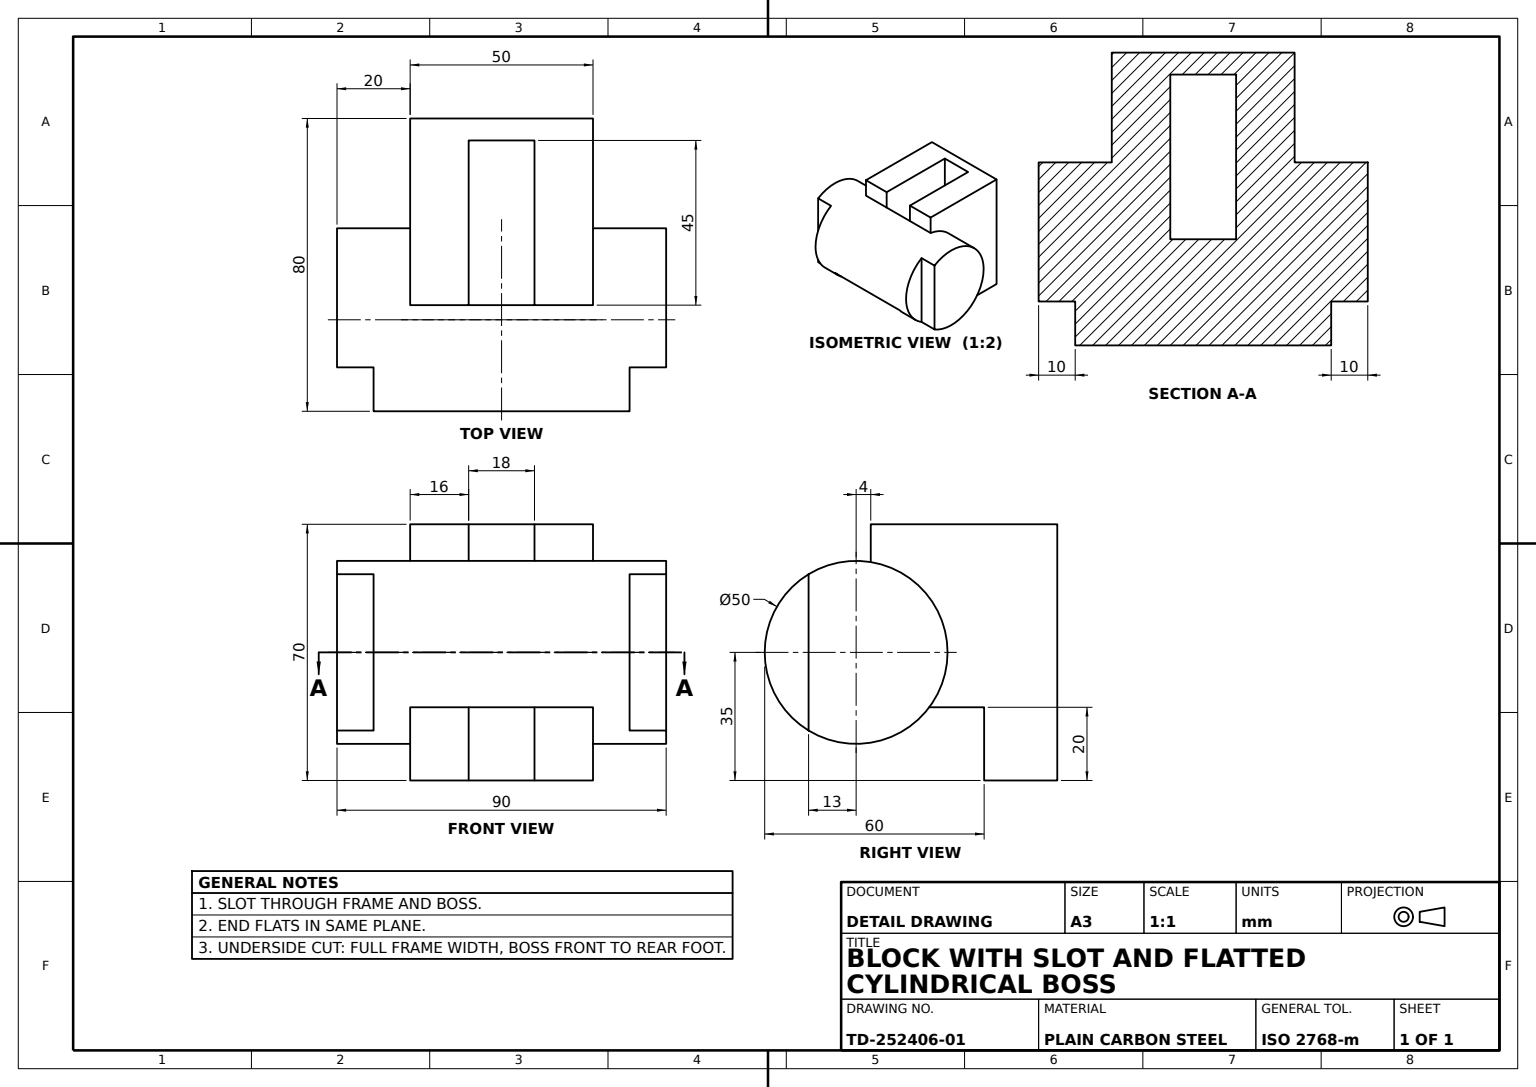
from build123d import *

# Parameters (mm, degrees)
BASE_PLATE_SKETCH_W         = 50
BASE_PLATE_SKETCH_H         = 70
BASE_PLATE_DEPTH            = 9
U_FRAME_SKETCH_W            = 16
U_FRAME_SKETCH_H            = 11
U_FRAME_DEPTH               = 70
SIDE_BLOCK_A_SKETCH_W       = 34
SIDE_BLOCK_A_SKETCH_H       = 50
SIDE_BLOCK_A_DEPTH          = 16
SIDE_BLOCK_B_SKETCH_W       = 34
SIDE_BLOCK_B_SKETCH_H       = 50
SIDE_BLOCK_B_DEPTH          = 16
BASE_RECESS_SKETCH_W        = 50
BASE_RECESS_SKETCH_H        = 70
BASE_RECESS_CUT_DEPTH       = 3
TOP_LIP_SKETCH_W            = 16
TOP_LIP_SKETCH_H            = 20
TOP_LIP_DEPTH               = 3
CYLINDER_SKETCH_R           = 25
CYLINDER_50_DEPTH           = 70
CYLINDER_START              = 20
CYLINDER_EXTENSION_SKETCH_R = 25
CYLINDER_EXTENSION_50_DEPTH = 20
U_SLOT_CUT_DEPTH            = 60
FRAME_CLEARANCE_SKETCH_W    = 18
FRAME_CLEARANCE_SKETCH_H    = 21
FRAME_CLEARANCE_CUT_DEPTH   = 50
END_FLAT_A_DEPTH            = 10
END_START                   = -10
END_FLAT_B_DEPTH            = 10


with BuildPart() as part:
    # Base Plate Sketch → Base Plate (new body)
    with BuildSketch(Plane.XY):
        with Locations((25, -35)):
            Rectangle(BASE_PLATE_SKETCH_W, BASE_PLATE_SKETCH_H)
    extrude(amount=BASE_PLATE_DEPTH)

    # U-Frame Sketch → U-Frame (add)
    with BuildSketch(Plane.XZ.offset(70)):
        with Locations((8, 14.5)):
            Rectangle(U_FRAME_SKETCH_W, U_FRAME_SKETCH_H)
        with Locations((42, 14.5)):
            Rectangle(U_FRAME_SKETCH_W, U_FRAME_SKETCH_H)
    extrude(amount=-U_FRAME_DEPTH)

    # Side Block A Sketch → Side Block A (add)
    with BuildSketch(Plane.ZY):
        with Locations((37, -25)):
            Rectangle(SIDE_BLOCK_A_SKETCH_W, SIDE_BLOCK_A_SKETCH_H)
    extrude(amount=-SIDE_BLOCK_A_DEPTH)

    # Side Block B Sketch → Side Block B (add)
    with BuildSketch(Plane(origin=(50, 0, 0), x_dir=(0, 0, -1), z_dir=(1, 0, 0))):
        with Locations((-37, -25)):
            Rectangle(SIDE_BLOCK_B_SKETCH_W, SIDE_BLOCK_B_SKETCH_H)
    extrude(amount=-SIDE_BLOCK_B_DEPTH)

    # Base Recess Sketch → Base Recess Cut (cut)
    with BuildSketch(Plane(origin=(0, 0, 0), x_dir=(-1, 0, 0), z_dir=(0, 0, -1))):
        with Locations((-25, -35)):
            Rectangle(BASE_RECESS_SKETCH_W, BASE_RECESS_SKETCH_H)
    extrude(amount=-BASE_RECESS_CUT_DEPTH, mode=Mode.SUBTRACT)

    # Top Lip Sketch → Top Lip (add)
    with BuildSketch(Plane.XY.offset(20)):
        with Locations((8, -60)):
            Rectangle(TOP_LIP_SKETCH_W, TOP_LIP_SKETCH_H)
        with Locations((42, -60)):
            Rectangle(TOP_LIP_SKETCH_W, TOP_LIP_SKETCH_H)
    extrude(amount=TOP_LIP_DEPTH)

    # Cylinder Sketch → Cylinder Ø50 (add)
    with BuildSketch(Plane.ZY):
        with Locations((58, -35)):
            Circle(CYLINDER_SKETCH_R)
    extrude(amount=-CYLINDER_50_DEPTH)

    # Cylinder Extension Sketch → Cylinder Extension Ø50 (add)
    with BuildSketch(Plane.ZY.offset(CYLINDER_START)):
        with Locations((58, -35)):
            Circle(CYLINDER_EXTENSION_SKETCH_R)
    extrude(amount=-CYLINDER_EXTENSION_50_DEPTH)

    # U-Slot Sketch → U-Slot Cut (cut)
    with BuildSketch(Plane.XY.offset(23)):
        Polygon((34, -70), (50, -70), (50, -50), (0, -50), (0, -70), align=None)
    extrude(amount=U_SLOT_CUT_DEPTH, mode=Mode.SUBTRACT)

    # Frame Clearance Sketch → Frame Clearance Cut (cut)
    with BuildSketch(Plane.XZ.offset(50)):
        with Locations((25, 43.5)):
            Rectangle(FRAME_CLEARANCE_SKETCH_W, FRAME_CLEARANCE_SKETCH_H)
    extrude(amount=-FRAME_CLEARANCE_CUT_DEPTH, mode=Mode.SUBTRACT)

    # End Flat A Sketch → End Flat A (cut)
    with BuildSketch(Plane.ZY.offset(20)):
        with BuildLine():
            Line((71, -13.645843496), (71, -56.354156504))
            ThreePointArc((71, -56.354156504), (83, -35), (71, -13.645843496))
        make_face()
    extrude(amount=-END_FLAT_A_DEPTH, mode=Mode.SUBTRACT)

    # End Flat B Sketch → End Flat B (cut)
    with BuildSketch(Plane(origin=(70, 0, 0), x_dir=(0, 0, -1), z_dir=(1, 0, 0)).offset(END_START)):
        with BuildLine():
            Line((-71, -13.645843496), (-71, -56.354156504))
            ThreePointArc((-71, -56.354156504), (-83, -35), (-71, -13.645843496))
        make_face()
    extrude(amount=END_FLAT_B_DEPTH, mode=Mode.SUBTRACT)


solid = part.part
